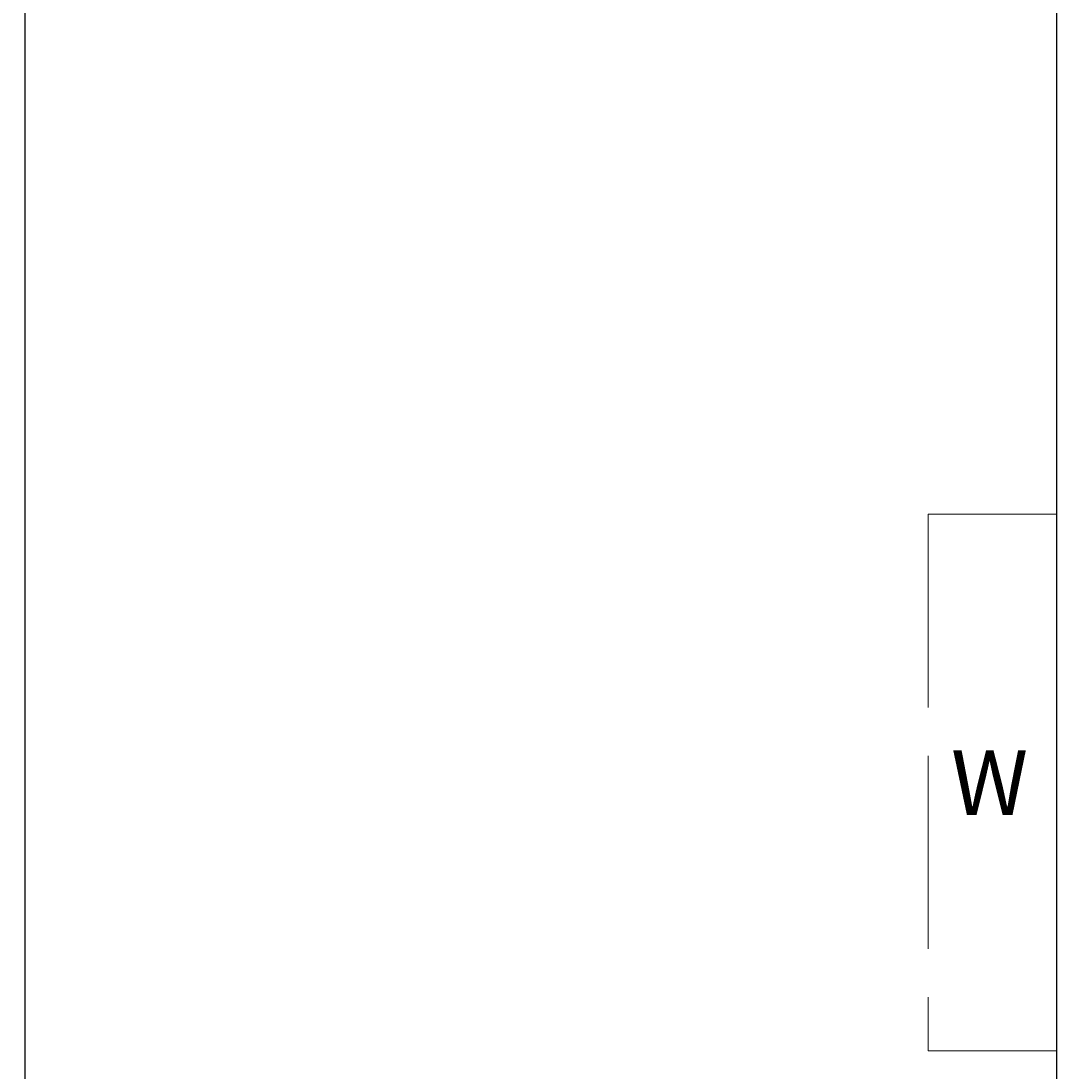
# Model space of a CAD drawing. Units: inches. Extents: x -301 to 715, y -607 to 364.
# Tile 53 of 141: x -301 to -205, y -171 to -73. Entities that reach past the tile are written whole.
import ezdxf

# ---------------------------------------------------------------- set-up
doc = ezdxf.new("R2010")
doc.units = ezdxf.units.IN
doc.header["$MEASUREMENT"] = 0
doc.linetypes.add('ACAD_ISO02W100', pattern=[15, 12, -3])
for name, color, linetype, lineweight in [('A-ANNO-DIMS', 2, 'Continuous', 18), ('A-ANNO-TEXT', 4, 'Continuous', 18), ('A-GLAZ-OVHD', 2, 'ACAD_ISO02W100', 18)]:
    doc.layers.add(name, color=color, linetype=linetype, lineweight=lineweight)
doc.styles.get("Standard").update_dxf_attribs({"font": 'arial.ttf'})
doc.dimstyles.get("Standard").update_dxf_attribs({"dimtxt": 0.18, "dimasz": 0.18, "dimexe": 0.18, "dimexo": 0.0625, "dimgap": 0.09, "dimtad": 0, "dimtih": 1, "dimtoh": 1, "dimdec": 1, "dimzin": 0, "dimdsep": 46, "dimlunit": 4, "dimtxsty": 'Standard', "dimcen": 0.09, "dimclrd": 3, "dimclre": 4, "dimclrt": 6, "dimadec": 0, "dimazin": 0, "dimtfac": 1, "dimtdec": 1, "dimtofl": 0, "dimtmove": 0, "dimatfit": 3, "dimfxl": 1, "dimtfill": 2, "dimtfillclr": 51, "dimtolj": 1, "dimtzin": 0, "dimarcsym": 0})

# ---------------------------------------------------------------- blocks, each defined once
blk = doc.blocks.new('WIN-SHADE-50')
at = {"ltscale": 1.5}
for p, q in [((0, 0), (0, 12)), ((50, 12), (0, 12)), ((50, 0), (50, 12)), ((5, 0), (0, 0)), ((45, 0), (50, 0))]:
    blk.add_line(p, q, dxfattribs=at)
blk = doc.blocks.new('*D145')
at = {"layer": 'A-ANNO-DIMS', "color": 4, "lineweight": -2, "transparency": 16777216}
for p, q in [((-204.666, 310.182), (-300.87, 310.182)), ((-204.666, -223.818), (-300.87, -223.818))]:
    blk.add_line(p, q, dxfattribs=at)
at = {"layer": 'A-ANNO-DIMS', "color": 3, "lineweight": -2, "transparency": 16777216}
for p, q in [((-300.69, 310.002), (-300.69, 43.364)), ((-300.69, -223.638), (-300.69, 43))]:
    blk.add_line(p, q, dxfattribs=at)
at = {"layer": 'A-ANNO-DIMS', "color": 3, "transparency": 16777216}
for points in [[(-300.72, 310.002), (-300.66, 310.002), (-300.69, 310.182)], [(-300.72, -223.638), (-300.66, -223.638), (-300.69, -223.818)]]:
    blk.add_solid(points, dxfattribs=at)
at = {"layer": 'Defpoints', "color": 0, "transparency": 16777216}
for p in [(-300.69, 310.182), (-204.603, 310.182), (-204.603, -223.818)]:
    blk.add_point(p, dxfattribs=at)
at = {"layer": 'A-ANNO-DIMS', "color": 6, "transparency": 16777216, "insert": (-300.69, 43.182), "char_height": 0.18, "attachment_point": 5, "bg_fill": 1, "box_fill_scale": 1.25, "bg_fill_color": 51, "bg_fill_transparency": 0}
blk.add_mtext('\\A1;44\'-6"', dxfattribs=at)
blk = doc.blocks.new('*D151')
at = {"layer": 'A-ANNO-DIMS', "color": 4, "lineweight": -2, "transparency": 16777216}
for p, q in [((-204.603, -223.755), (-204.603, 359.612)), ((-45.603, -214.755), (-45.603, 359.612))]:
    blk.add_line(p, q, dxfattribs=at)
at = {"layer": 'A-ANNO-DIMS', "color": 3, "lineweight": -2, "transparency": 16777216}
for p, q in [((-204.423, 359.432), (-125.494, 359.432)), ((-45.783, 359.432), (-124.713, 359.432))]:
    blk.add_line(p, q, dxfattribs=at)
at = {"layer": 'A-ANNO-DIMS', "color": 3, "transparency": 16777216}
for points in [[(-204.423, 359.462), (-204.423, 359.402), (-204.603, 359.432)], [(-45.783, 359.462), (-45.783, 359.402), (-45.603, 359.432)]]:
    blk.add_solid(points, dxfattribs=at)
at = {"layer": 'Defpoints', "color": 0, "transparency": 16777216}
for p in [(-45.603, 359.432), (-45.603, -214.818), (-204.603, -223.818)]:
    blk.add_point(p, dxfattribs=at)
at = {"layer": 'A-ANNO-DIMS', "color": 6, "transparency": 16777216, "insert": (-125.103, 359.432), "char_height": 0.18, "attachment_point": 5, "bg_fill": 1, "box_fill_scale": 1.25, "bg_fill_color": 51, "bg_fill_transparency": 0}
blk.add_mtext('\\A1;13\'-3"', dxfattribs=at)

msp = doc.modelspace()

# ---------------------------------------------------------------- block references
at = {"layer": 'A-GLAZ-OVHD', "rotation": 90.00000000000011}
msp.add_blockref('WIN-SHADE-50', (-204.603, -169.067), dxfattribs=at)

# ---------------------------------------------------------------- texts
at = {"layer": 'A-ANNO-TEXT'}
msp.add_text('W', height=6, dxfattribs=at).set_placement((-214.475, -147.083))

# ---------------------------------------------------------------- dimensions: what is measured, and where the dimension line sits
at = {"layer": 'A-ANNO-DIMS'}
dim = msp.add_linear_dim(base=(-45.603, 359.432), p1=(-204.603, -223.818), p2=(-45.603, -214.818), dimstyle='Standard', override={"dimdec": 1, "dimlfac": 1, "dimrnd": 0, "dimzin": 1, "dimdsep": 46, "dimlunit": 4, "dimfrac": 2}, dxfattribs=at)
dim.commit()
dim.dimension.update_dxf_attribs({"geometry": '*D151', "text_midpoint": (-125.103, 359.432)})
dim = msp.add_linear_dim(base=(-300.69, 310.182), p1=(-204.603, -223.818), p2=(-204.603, 310.182), angle=90, dimstyle='Standard', override={"dimdec": 1, "dimlfac": 1, "dimrnd": 0, "dimzin": 1, "dimdsep": 46, "dimlunit": 4, "dimfrac": 2}, dxfattribs=at)
dim.commit()
dim.dimension.update_dxf_attribs({"geometry": '*D145', "text_midpoint": (-300.69, 43.182)})

doc.saveas('drawing.dxf')
